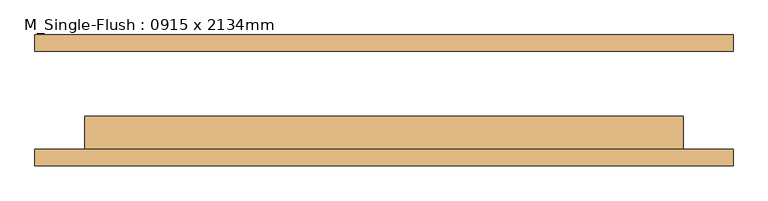
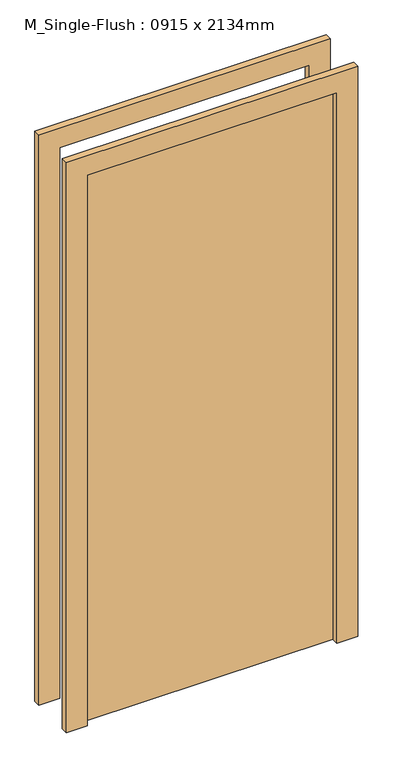
"""IFC4 building model written with IfcOpenShell, lengths in millimetres: door geometry, M_Single-Flush : 0915 x 2134mm."""

from ifc_helpers import new_model, si_unit, frame, origin, origin_with_axes, place, context, project, spatial, polyline, outline, extrude, source, transform, mapped, element, save


def m_single_flush_0915_x_2134mm_f3d7f739(model_context):
    return source(origin(), model_context, "Body", "SweptSolid", [
        extrude(outline(polyline([(2210.0, -533.5), (0.0, -533.5), (0.0, -457.5), (2134.0, -457.5), (2134.0, 457.5), (0.0, 457.5), (0.0, 533.5), (2210.0, 533.5), (2210.0, -533.5)])), frame((0.0, -100.0, 0.0), z_axis=(0.0, 1.0, 0.0), x_axis=(0.0, 0.0, 1.0)), (0.0, 0.0, 1.0), 25.0),
        extrude(outline(polyline([(2210.0, 533.5), (2210.0, -533.5), (0.0, -533.5), (0.0, -457.5), (2134.0, -457.5), (2134.0, 457.5), (0.0, 457.5), (0.0, 533.5), (2210.0, 533.5)])), frame((0.0, 75.0, 0.0), z_axis=(0.0, 1.0, 0.0), x_axis=(0.0, 0.0, 1.0)), (0.0, 0.0, 1.0), 25.0),
        extrude(outline(polyline([(457.5, -24.0), (457.5, -75.0), (-457.5, -75.0), (-457.5, -24.0), (457.5, -24.0)])), origin_with_axes(), (0.0, 0.0, 1.0), 2134.0),
    ])


if __name__ == "__main__":
    model = new_model("IFC4")
    model_context = context("Model", 3, world=origin())
    ifc_project = project(units=[si_unit("LENGTHUNIT", "METRE", prefix="MILLI")], contexts=[model_context])
    site = spatial("IfcSite", under=ifc_project)
    building = spatial("IfcBuilding", under=site)
    placement = place(None, origin())
    m_single_flush_0915_x_2134mm_shape = m_single_flush_0915_x_2134mm_f3d7f739(model_context)
    element("IfcDoor", 1, ObjectType="M_Single-Flush : 0915 x 2134mm", at=placement, inside=building, context=model_context, shape_type="MappedRepresentation", body=[
        mapped(m_single_flush_0915_x_2134mm_shape, transform((0.0, 0.0, 0.0), x_axis=(1.0, 0.0, 0.0), y_axis=(0.0, 1.0, 0.0), z_axis=(0.0, 0.0, 1.0))),
    ])
    save(model, "model.ifc")

# Revit data of these elements
# Type "M_Single-Flush : 0915 x 2134mm"
#   Type Mark = "20"
#   Construction Type Id = "MDOOR"
#   Analytic Construction = "Metal"
#   Thickness = 0.051 m
#   Thermal Resistance (R) = 0.270117 (m²·K)/W
#   Heat Transfer Coefficient (U) = 3.7021 W/(m²·K)
#   Height = 2.134 m
#   Trim Projection Ext = 0.025 m
#   Trim Projection Int = 0.025 m
#   Trim Width = 0.076 m
#   Width = 0.915 m
#   Define Thermal Properties by = 1
#   Define Thermal Properties by = 1
#   Door Material = Door - Panel
#   Frame Material = Door - Frame
#   Visual Light Transmittance = 0
#   Solar Heat Gain Coefficient = 0
#   Function = (empty or 0)
#   Wall Closure = (empty or 0)
# Element 1 (IfcDoor, "M_Single-Flush : 0915 x 2134mm")
#   Materials on its faces: "Door - Frame", "Door - Panel"
# Materials
#   "Door - Panel": class "Wood", colour RGB 210 159 95, transparency 0, Cost = 0
#   "Door - Frame": colour RGB 118 70 51, transparency 0, Cost = 0
